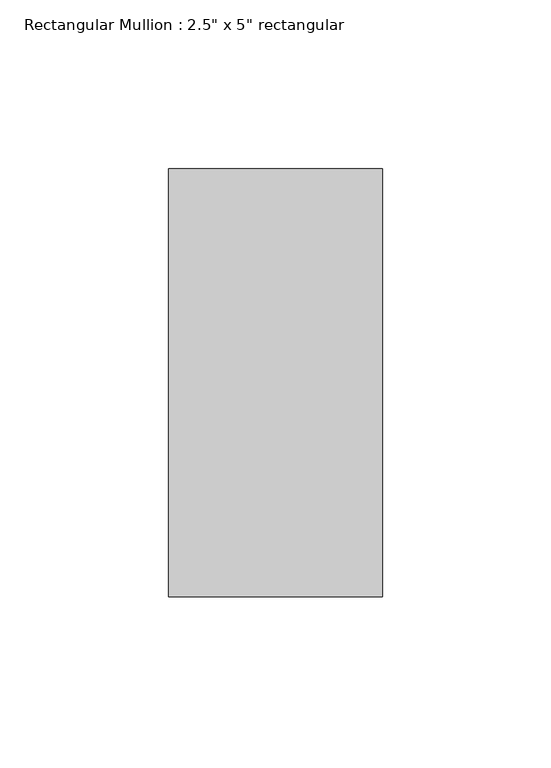
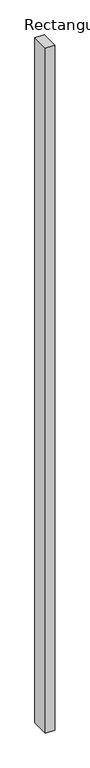
"""IFC4 building model written with IfcOpenShell, lengths in millimetres: member geometry."""

from ifc_helpers import new_model, si_unit, frame, origin, place, context, project, spatial, polyline, outline, extrude, source, transform, mapped, element, save


def member_9fca3acb(model_context):
    return source(origin(), model_context, "Body", "SweptSolid", [
        extrude(outline(polyline([(0.0, 63.5), (0.0, -63.5), (-63.5, -63.5), (-63.5, 63.5), (0.0, 63.5)])), frame((0.0, 0.0, -5013.5306476), z_axis=(0.0, 0.0, 1.0), x_axis=(1.0, 0.0, 0.0)), (0.0, 0.0, 1.0), 5013.5306476),
    ])


if __name__ == "__main__":
    model = new_model("IFC4")
    model_context = context("Model", 3, world=origin())
    ifc_project = project(units=[si_unit("LENGTHUNIT", "METRE", prefix="MILLI")], contexts=[model_context])
    site = spatial("IfcSite", under=ifc_project)
    building = spatial("IfcBuilding", under=site)
    placement = place(None, origin())
    member_shape = member_9fca3acb(model_context)
    element("IfcMember", 1, ObjectType="Rectangular Mullion : 2.5\" x 5\" rectangular", at=placement, inside=building, context=model_context, shape_type="MappedRepresentation", body=[
        mapped(member_shape, transform((0.0, 0.0, 0.0), x_axis=(1.0, 0.0, 0.0), y_axis=(0.0, 1.0, 0.0), z_axis=(0.0, 0.0, 1.0))),
    ])
    save(model, "model.ifc")

# Revit data of these elements
# Type "Rectangular Mullion : 2.5\" x 5\" rectangular"
#   built-in parameter 1007304 = 0.416667 (stored number, unit not read)
#   built-in parameter 1007301 = 0.104167 (stored number, unit not read)
#   built-in parameter 1007300 = 0.104167 (stored number, unit not read)
# Element 1 (IfcMember, "Rectangular Mullion : 2.5\" x 5\" rectangular")
#   Materials on its faces: "Aluminum"
# Materials
#   "Aluminum": class "Metal", colour RGB 247 247 247, transparency 0, Description = "Aluminum 6061", Cost = 0
